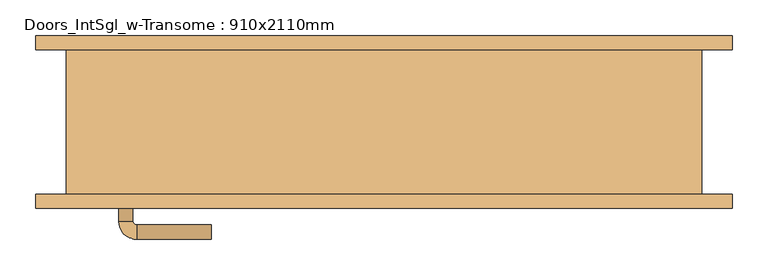
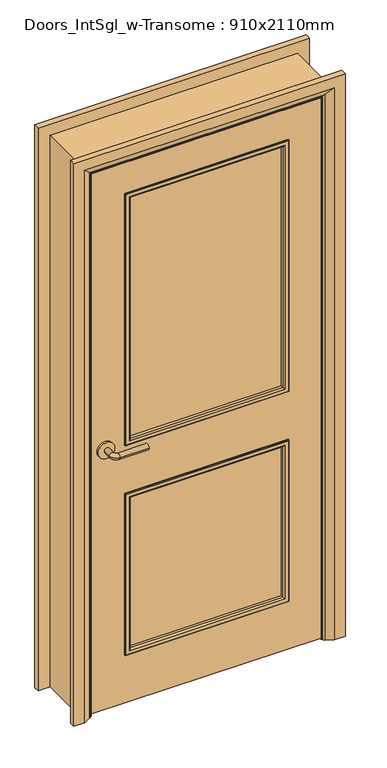
"""IFC4 building model written with IfcOpenShell, lengths in millimetres: door geometry, Doors_IntSgl_w-Transome : 910x2110mm."""

from ifc_helpers import new_model, si_unit, point, frame, frame_2d, origin, place, context, project, spatial, polyline, circle_curve, ellipse_curve, trimmed, segment, composite_curve, outline, extrude, faceted_brep, source, transform, mapped, element, save
from ifc_brep_helpers import plane_surface, cylinder_surface, revolved_surface, advanced_brep


def doors_intsgl_w_transome_910x2110mm_1071bad6(model_context):
    return source(origin(), model_context, "Body", "SolidModel", [
        advanced_brep(
        [(-373.0, -55.6, 1000.0), (-353.0, -55.6, 1000.0), (-373.0, -25.6, 1000.0), (-353.0, -25.6, 1000.0), (-348.0, -20.6, 1000.0), (-348.0, -0.6, 1000.0), (-243.0, -0.6, 1000.0), (-243.0, -20.6, 1000.0)],
        [
            (0, 1, circle_curve(frame((-363.0, -55.6, 1000.0), z_axis=(0.0, -1.0, 0.0), x_axis=(1.0, 0.0, 0.0)), 10.0)),
            (1, 0, circle_curve(frame((-363.0, -55.6, 1000.0), z_axis=(0.0, -1.0, 0.0), x_axis=(1.0, 0.0, 0.0)), 10.0)),
            (0, 2),
            (2, 3, circle_curve(frame((-363.0, -25.6, 1000.0), z_axis=(0.0, -1.0, 0.0), x_axis=(1.0, 0.0, 0.0)), 10.0)),
            (3, 1),
            (3, 2, circle_curve(frame((-363.0, -25.6, 1000.0), z_axis=(0.0, -1.0, 0.0), x_axis=(1.0, 0.0, 0.0)), 10.0)),
            (4, 3, circle_curve(frame((-348.0, -25.6, 1000.0), z_axis=(0.0, 0.0, 1.0), x_axis=(-1.0, 0.0, 0.0)), 5.0)),
            (2, 5, circle_curve(frame((-348.0, -25.6, 1000.0), z_axis=(0.0, 0.0, -1.0), x_axis=(-1.0, 0.0, 0.0)), 25.0)),
            (5, 4, circle_curve(frame((-348.0, -10.6, 1000.0), z_axis=(-1.0, 0.0, 0.0), x_axis=(0.0, -1.0, 0.0)), 10.0)),
            (4, 5, circle_curve(frame((-348.0, -10.6, 1000.0), z_axis=(-1.0, 0.0, 0.0), x_axis=(0.0, -1.0, 0.0)), 10.0)),
            (6, 7, circle_curve(frame((-243.0, -10.6, 1000.0), z_axis=(1.0, 0.0, 0.0), x_axis=(0.0, -1.0, 0.0)), 10.0)),
            (7, 6, circle_curve(frame((-243.0, -10.6, 1000.0), z_axis=(1.0, 0.0, 0.0), x_axis=(0.0, -1.0, 0.0)), 10.0)),
            (5, 6),
            (7, 4),
        ],
        [
            plane_surface(frame((-363.0, -55.6, 1000.0), z_axis=(0.0, -1.0, 0.0), x_axis=(0.0, 0.0, 1.0))),
            cylinder_surface(frame((-363.0, -55.6, 1000.0), z_axis=(0.0, -1.0, 0.0), x_axis=(1.0, 0.0, 0.0)), 10.0),
            revolved_surface(trimmed(ellipse_curve(frame((-363.0, -25.6, 1000.0), z_axis=(0.0, -1.0, 0.0), x_axis=(1.0, 0.0, 0.0)), 10.0, 10.0), [point((-373.0, -25.6, 1000.0))], [point((-353.0, -25.6, 1000.0))], True, "CARTESIAN"), (-348.0, -25.6, 1000.0), (0.0, 0.0, -1.0)),
            revolved_surface(trimmed(ellipse_curve(frame((-363.0, -25.6, 1000.0), z_axis=(0.0, -1.0, 0.0), x_axis=(1.0, 0.0, 0.0)), 10.0, 10.0), [point((-353.0, -25.6, 1000.0))], [point((-373.0, -25.6, 1000.0))], True, "CARTESIAN"), (-348.0, -25.6, 1000.0), (0.0, 0.0, -1.0)),
            plane_surface(frame((-243.0, -10.6, 1000.0), z_axis=(1.0, 0.0, 0.0), x_axis=(0.0, 0.0, 1.0))),
            cylinder_surface(frame((-348.0, -10.6, 1000.0), z_axis=(-1.0, 0.0, 0.0), x_axis=(0.0, -1.0, 0.0)), 10.0),
        ],
        [
            (0, [[1, 2]]),
            (1, [[-1, 3, 4, 5]]),
            (1, [[-2, -5, 6, -3]]),
            (2, [[7, -4, 8, 9]]),
            (3, [[-8, -6, -7, 10]]),
            (4, [[11, 12]]),
            (5, [[-9, 13, -12, 14]]),
            (5, [[-10, -14, -11, -13]]),
        ],
    ),
        extrude(outline(composite_curve([segment(trimmed(circle_curve(frame_2d((1000.0, -365.5)), 30.0), [point((1000.0, -395.5))], [point((1000.0, -335.5))], False, "CARTESIAN"), True, "CONTINUOUS"), segment(trimmed(circle_curve(frame_2d((1000.0, -365.5)), 30.0), [point((1000.0, -335.5))], [point((1000.0, -395.5))], False, "CARTESIAN"), True, "CONTINUOUS")], self_intersect=False)), frame((0.0, -63.6, 0.0), z_axis=(0.0, 1.0, 0.0), x_axis=(0.0, 0.0, 1.0)), (0.0, 0.0, 1.0), 8.0),
        advanced_brep(
        [(-373.0, -109.6, 1000.0), (-353.0, -109.6, 1000.0), (-353.0, -139.6, 1000.0), (-373.0, -139.6, 1000.0), (-348.0, -144.6, 1000.0), (-348.0, -164.6, 1000.0), (-243.0, -164.6, 1000.0), (-243.0, -144.6, 1000.0)],
        [
            (0, 1, circle_curve(frame((-363.0, -109.6, 1000.0), z_axis=(0.0, 1.0, 0.0), x_axis=(1.0, 0.0, 0.0)), 10.0)),
            (1, 0, circle_curve(frame((-363.0, -109.6, 1000.0), z_axis=(0.0, 1.0, 0.0), x_axis=(1.0, 0.0, 0.0)), 10.0)),
            (1, 2),
            (2, 3, circle_curve(frame((-363.0, -139.6, 1000.0), z_axis=(0.0, 1.0, 0.0), x_axis=(1.0, 0.0, 0.0)), 10.0)),
            (3, 0),
            (3, 2, circle_curve(frame((-363.0, -139.6, 1000.0), z_axis=(0.0, 1.0, 0.0), x_axis=(1.0, 0.0, 0.0)), 10.0)),
            (4, 5, circle_curve(frame((-348.0, -154.6, 1000.0), z_axis=(-1.0, 0.0, 0.0), x_axis=(0.0, 1.0, 0.0)), 10.0)),
            (5, 3, circle_curve(frame((-348.0, -139.6, 1000.0), z_axis=(0.0, 0.0, -1.0), x_axis=(-1.0, 0.0, 0.0)), 25.0)),
            (2, 4, circle_curve(frame((-348.0, -139.6, 1000.0), z_axis=(0.0, 0.0, 1.0), x_axis=(-1.0, 0.0, 0.0)), 5.0)),
            (5, 4, circle_curve(frame((-348.0, -154.6, 1000.0), z_axis=(-1.0, 0.0, 0.0), x_axis=(0.0, 1.0, 0.0)), 10.0)),
            (6, 7, circle_curve(frame((-243.0, -154.6, 1000.0), z_axis=(1.0, 0.0, 0.0), x_axis=(0.0, 1.0, 0.0)), 10.0)),
            (7, 6, circle_curve(frame((-243.0, -154.6, 1000.0), z_axis=(1.0, 0.0, 0.0), x_axis=(0.0, 1.0, 0.0)), 10.0)),
            (4, 7),
            (6, 5),
        ],
        [
            plane_surface(frame((-363.0, -109.6, 1000.0), z_axis=(0.0, 1.0, 0.0), x_axis=(0.0, 0.0, 1.0))),
            cylinder_surface(frame((-363.0, -109.6, 1000.0), z_axis=(0.0, 1.0, 0.0), x_axis=(1.0, 0.0, 0.0)), 10.0),
            revolved_surface(trimmed(ellipse_curve(frame((-363.0, -139.6, 1000.0), z_axis=(0.0, -1.0, 0.0), x_axis=(1.0, 0.0, 0.0)), 10.0, 10.0), [point((-373.0, -139.6, 1000.0))], [point((-353.0, -139.6, 1000.0))], True, "CARTESIAN"), (-348.0, -139.6, 1000.0), (0.0, 0.0, -1.0)),
            revolved_surface(trimmed(ellipse_curve(frame((-363.0, -139.6, 1000.0), z_axis=(0.0, -1.0, 0.0), x_axis=(1.0, 0.0, 0.0)), 10.0, 10.0), [point((-353.0, -139.6, 1000.0))], [point((-373.0, -139.6, 1000.0))], True, "CARTESIAN"), (-348.0, -139.6, 1000.0), (0.0, 0.0, -1.0)),
            plane_surface(frame((-243.0, -154.6, 1000.0), z_axis=(1.0, 0.0, 0.0), x_axis=(0.0, 0.0, 1.0))),
            cylinder_surface(frame((-348.0, -154.6, 1000.0), z_axis=(-1.0, 0.0, 0.0), x_axis=(0.0, 1.0, 0.0)), 10.0),
        ],
        [
            (0, [[1, 2]]),
            (1, [[3, 4, 5, -2]]),
            (1, [[-5, 6, -3, -1]]),
            (2, [[7, 8, -4, 9]]),
            (3, [[10, -9, -6, -8]]),
            (4, [[11, 12]]),
            (5, [[13, -11, 14, -7]]),
            (5, [[-14, -12, -13, -10]]),
        ],
    ),
        extrude(outline(composite_curve([segment(trimmed(circle_curve(frame_2d((1000.0, -365.5)), 30.0), [point((1000.0, -395.5))], [point((1000.0, -335.5))], False, "CARTESIAN"), True, "CONTINUOUS"), segment(trimmed(circle_curve(frame_2d((1000.0, -365.5)), 30.0), [point((1000.0, -335.5))], [point((1000.0, -395.5))], False, "CARTESIAN"), True, "CONTINUOUS")], self_intersect=False)), frame((0.0, -109.6, 0.0), z_axis=(0.0, 1.0, 0.0), x_axis=(0.0, 0.0, 1.0)), (0.0, 0.0, 1.0), 8.0),
        extrude(outline(polyline([(2068.0, -413.0), (8.0, -413.0), (8.0, 413.0), (2068.0, 413.0), (2068.0, -413.0)]), holes=[polyline([(1943.0, 288.0), (1000.0, 288.0), (1000.0, -288.0), (1943.0, -288.0), (1943.0, 288.0)]), polyline([(800.0, -288.0), (800.0, 288.0), (200.0, 288.0), (200.0, -288.0), (800.0, -288.0)])]), frame((0.0, -101.6, 0.0), z_axis=(0.0, 1.0, 0.0), x_axis=(0.0, 0.0, 1.0)), (0.0, 0.0, 1.0), 38.0),
        extrude(outline(polyline([(-288.0, -91.6), (-288.0, -73.6), (288.0, -73.6), (288.0, -91.6), (-288.0, -91.6)])), frame((0.0, 0.0, 1000.0), z_axis=(0.0, 0.0, 1.0), x_axis=(1.0, 0.0, 0.0)), (0.0, 0.0, 1.0), 943.0),
        extrude(outline(polyline([(-288.0, -91.6), (-288.0, -73.6), (288.0, -73.6), (288.0, -91.6), (-288.0, -91.6)])), frame((0.0, 0.0, 200.0), z_axis=(0.0, 0.0, 1.0), x_axis=(1.0, 0.0, 0.0)), (0.0, 0.0, 1.0), 600.0),
        faceted_brep([(-415.0, -101.6, 0.0), (-447.0, -101.6, 0.0), (-447.0, 101.6, 0.0), (-415.0, 101.6, 0.0), (-415.0, 101.6, 2070.0), (-415.0, -101.6, 2070.0), (-447.0, 101.6, 2102.0), (-447.0, -101.6, 2102.0), (415.0, -101.6, 0.0), (415.0, 101.6, 0.0), (447.0, 101.6, 0.0), (447.0, -101.6, 0.0), (415.0, -101.6, 2070.0), (447.0, -101.6, 2102.0), (447.0, 101.6, 2102.0), (415.0, 101.6, 2070.0)], [[[0, 1, 2, 3]], [[3, 4, 5, 0]], [[2, 6, 4, 3]], [[1, 7, 6, 2]], [[0, 5, 7, 1]], [[8, 9, 10, 11]], [[12, 8, 11, 13]], [[13, 11, 10, 14]], [[14, 10, 9, 15]], [[15, 9, 8, 12]], [[4, 15, 12, 5]], [[6, 14, 15, 4]], [[7, 13, 14, 6]], [[5, 12, 13, 7]]]),
        extrude(outline(polyline([(0.0, -396.0), (2051.0, -396.0), (2051.0, 396.0), (0.0, 396.0), (0.0, 415.0), (2070.0, 415.0), (2070.0, -415.0), (0.0, -415.0), (0.0, -396.0)])), frame((0.0, -61.6, 0.0), z_axis=(0.0, 1.0, 0.0), x_axis=(0.0, 0.0, 1.0)), (0.0, 0.0, 1.0), 32.0),
        advanced_brep(
        [(-490.0, 121.6, 0.0), (-450.0, 121.6, 0.0), (-424.0, 107.6, 0.0), (-420.0, 101.6, 0.0), (-490.0, 101.6, 0.0), (-490.0, 101.6, 2145.0), (-490.0, 121.6, 2145.0), (-420.0, 101.6, 2075.0), (420.0, 101.6, 2075.0), (420.0, 101.6, 0.0), (490.0, 101.6, 0.0), (490.0, 101.6, 2145.0), (-424.0, 107.6, 2079.0), (-450.0, 121.6, 2105.0), (490.0, 121.6, 2145.0), (490.0, 121.6, 0.0), (450.0, 121.6, 0.0), (450.0, 121.6, 2105.0), (424.0, 107.6, 0.0), (424.0, 107.6, 2079.0)],
        [
            (0, 1),
            (1, 2),
            (2, 3, circle_curve(frame((-428.0, 100.6, 0.0), z_axis=(0.0, 0.0, -1.0), x_axis=(-1.0, 0.0, 0.0)), 8.0622577)),
            (3, 4),
            (4, 0),
            (4, 5),
            (5, 6),
            (6, 0),
            (3, 7),
            (7, 8),
            (8, 9),
            (9, 10),
            (10, 11),
            (11, 5),
            (2, 12),
            (12, 7, ellipse_curve(frame((-428.0, 100.6, 2083.0), z_axis=(-0.7071067811865475, 0.0, -0.7071067811865475), x_axis=(0.7071067811865474, 0.0, -0.7071067811865476)), 11.4017543, 8.0622577)),
            (1, 13),
            (13, 12),
            (6, 14),
            (14, 15),
            (15, 16),
            (16, 17),
            (17, 13),
            (10, 15),
            (14, 11),
            (9, 18, circle_curve(frame((428.0, 100.6, 0.0), z_axis=(0.0, 0.0, -1.0), x_axis=(1.0, 0.0, 0.0)), 8.0622577)),
            (18, 16),
            (19, 18),
            (8, 19, ellipse_curve(frame((428.0, 100.6, 2083.0), z_axis=(0.7071067811865475, 0.0, -0.7071067811865475), x_axis=(0.7071067811865474, 0.0, 0.7071067811865476)), 11.4017543, 8.0622577)),
            (19, 17),
            (12, 19),
        ],
        [
            plane_surface(frame((-420.0, 101.6, 0.0), z_axis=(0.0, 0.0, -1.0), x_axis=(0.0, 1.0, 0.0))),
            plane_surface(frame((-490.0, 121.6, 0.0), z_axis=(-1.0, 0.0, 0.0), x_axis=(0.0, 0.0, 1.0))),
            plane_surface(frame((-490.0, 101.6, 0.0), z_axis=(0.0, -1.0, 0.0), x_axis=(0.0, 0.0, 1.0))),
            cylinder_surface(frame((-428.0, 100.6, 0.0), z_axis=(0.0, 0.0, -1.0), x_axis=(-1.0, 0.0, 0.0)), 8.0622577),
            plane_surface(frame((-424.0, 107.6, 0.0), z_axis=(0.4740998230350183, 0.8804710999221749, 0.0), x_axis=(0.0, 0.0, 1.0))),
            plane_surface(frame((-450.0, 121.6, 0.0), z_axis=(0.0, 1.0, 0.0), x_axis=(0.0, 0.0, 1.0))),
            plane_surface(frame((490.0, 121.6, 2145.0), z_axis=(1.0, 0.0, 0.0), x_axis=(0.0, 0.0, -1.0))),
            plane_surface(frame((420.0, 101.6, 0.0), z_axis=(0.0, 0.0, -1.0), x_axis=(0.0, 1.0, 0.0))),
            cylinder_surface(frame((428.0, 100.6, 2075.0), z_axis=(0.0, 0.0, 1.0), x_axis=(1.0, 0.0, 0.0)), 8.0622577),
            plane_surface(frame((424.0, 107.6, 2079.0), z_axis=(-0.4740998230350183, 0.8804710999221749, 0.0), x_axis=(0.0, 0.0, -1.0))),
            plane_surface(frame((-490.0, 121.6, 2145.0), z_axis=(0.0, 0.0, 1.0), x_axis=(1.0, 0.0, 0.0))),
            cylinder_surface(frame((-420.0, 100.6, 2083.0), z_axis=(-1.0, 0.0, 0.0), x_axis=(0.0, 0.0, 1.0)), 8.0622577),
            plane_surface(frame((-424.0, 107.6, 2079.0), z_axis=(0.0, 0.8804710999221749, -0.4740998230350183), x_axis=(1.0, 0.0, 0.0))),
        ],
        [
            (0, [[1, 2, 3, 4, 5]]),
            (1, [[6, 7, 8, -5]]),
            (2, [[9, 10, 11, 12, 13, 14, -6, -4]]),
            (3, [[15, 16, -9, -3]]),
            (4, [[17, 18, -15, -2]]),
            (5, [[-8, 19, 20, 21, 22, 23, -17, -1]]),
            (6, [[-13, 24, -20, 25]]),
            (7, [[-24, -12, 26, 27, -21]]),
            (8, [[28, -26, -11, 29]]),
            (9, [[-22, -27, -28, 30]]),
            (10, [[-14, -25, -19, -7]]),
            (11, [[31, -29, -10, -16]]),
            (12, [[-23, -30, -31, -18]]),
        ],
    ),
        advanced_brep(
        [(490.0, -121.6, 0.0), (450.0, -121.6, 0.0), (424.0, -107.6, 0.0), (420.0, -101.6, 0.0), (490.0, -101.6, 0.0), (490.0, -101.6, 2145.0), (490.0, -121.6, 2145.0), (420.0, -101.6, 2075.0), (-420.0, -101.6, 2075.0), (-420.0, -101.6, 0.0), (-490.0, -101.6, 0.0), (-490.0, -101.6, 2145.0), (424.0, -107.6, 2079.0), (450.0, -121.6, 2105.0), (-490.0, -121.6, 2145.0), (-490.0, -121.6, 0.0), (-450.0, -121.6, 0.0), (-450.0, -121.6, 2105.0), (-424.0, -107.6, 0.0), (-424.0, -107.6, 2079.0)],
        [
            (0, 1),
            (1, 2),
            (2, 3, circle_curve(frame((428.0, -100.6, 0.0), z_axis=(0.0, 0.0, -1.0), x_axis=(1.0, 0.0, 0.0)), 8.0622577)),
            (3, 4),
            (4, 0),
            (4, 5),
            (5, 6),
            (6, 0),
            (3, 7),
            (7, 8),
            (8, 9),
            (9, 10),
            (10, 11),
            (11, 5),
            (2, 12),
            (12, 7, ellipse_curve(frame((428.0, -100.6, 2083.0), z_axis=(0.7071067811865475, 0.0, -0.7071067811865475), x_axis=(-0.7071067811865474, 0.0, -0.7071067811865476)), 11.4017543, 8.0622577)),
            (1, 13),
            (13, 12),
            (6, 14),
            (14, 15),
            (15, 16),
            (16, 17),
            (17, 13),
            (10, 15),
            (14, 11),
            (9, 18, circle_curve(frame((-428.0, -100.6, 0.0), z_axis=(0.0, 0.0, -1.0), x_axis=(-1.0, 0.0, 0.0)), 8.0622577)),
            (18, 16),
            (19, 18),
            (8, 19, ellipse_curve(frame((-428.0, -100.6, 2083.0), z_axis=(-0.7071067811865475, 0.0, -0.7071067811865475), x_axis=(-0.7071067811865474, 0.0, 0.7071067811865476)), 11.4017543, 8.0622577)),
            (19, 17),
            (12, 19),
        ],
        [
            plane_surface(frame((420.0, -101.6, 0.0), z_axis=(0.0, 0.0, -1.0), x_axis=(0.0, 1.0, 0.0))),
            plane_surface(frame((490.0, -121.6, 0.0), z_axis=(1.0, 0.0, 0.0), x_axis=(0.0, 0.0, 1.0))),
            plane_surface(frame((490.0, -101.6, 0.0), z_axis=(0.0, 1.0, 0.0), x_axis=(0.0, 0.0, 1.0))),
            cylinder_surface(frame((428.0, -100.6, 0.0), z_axis=(0.0, 0.0, -1.0), x_axis=(1.0, 0.0, 0.0)), 8.0622577),
            plane_surface(frame((424.0, -107.6, 0.0), z_axis=(-0.4740998230350126, -0.880471099922178, 0.0), x_axis=(0.0, 0.0, 1.0))),
            plane_surface(frame((450.0, -121.6, 0.0), z_axis=(0.0, -1.0, 0.0), x_axis=(0.0, 0.0, 1.0))),
            plane_surface(frame((-490.0, -121.6, 2145.0), z_axis=(-1.0, 0.0, 0.0), x_axis=(0.0, 0.0, -1.0))),
            plane_surface(frame((-420.0, -101.6, 0.0), z_axis=(0.0, 0.0, -1.0), x_axis=(0.0, 1.0, 0.0))),
            cylinder_surface(frame((-428.0, -100.6, 2075.0), z_axis=(0.0, 0.0, 1.0), x_axis=(-1.0, 0.0, 0.0)), 8.0622577),
            plane_surface(frame((-424.0, -107.6, 2079.0), z_axis=(0.47409982303501824, -0.8804710999221749, 0.0), x_axis=(0.0, 0.0, -1.0))),
            plane_surface(frame((490.0, -121.6, 2145.0), z_axis=(0.0, 0.0, 1.0), x_axis=(-1.0, 0.0, 0.0))),
            cylinder_surface(frame((420.0, -100.6, 2083.0), z_axis=(1.0, 0.0, 0.0), x_axis=(0.0, 0.0, 1.0)), 8.0622577),
            plane_surface(frame((424.0, -107.6, 2079.0), z_axis=(0.0, -0.8804710999221764, -0.4740998230350154), x_axis=(-1.0, 0.0, 0.0))),
        ],
        [
            (0, [[1, 2, 3, 4, 5]]),
            (1, [[6, 7, 8, -5]]),
            (2, [[9, 10, 11, 12, 13, 14, -6, -4]]),
            (3, [[15, 16, -9, -3]]),
            (4, [[17, 18, -15, -2]]),
            (5, [[-8, 19, 20, 21, 22, 23, -17, -1]]),
            (6, [[-13, 24, -20, 25]]),
            (7, [[-24, -12, 26, 27, -21]]),
            (8, [[28, -26, -11, 29]]),
            (9, [[-22, -27, -28, 30]]),
            (10, [[-14, -25, -19, -7]]),
            (11, [[31, -29, -10, -16]]),
            (12, [[-23, -30, -31, -18]]),
        ],
    ),
        advanced_brep(
        [(-288.0, -91.6, 1943.0), (-288.0, -91.6, 1000.0), (-288.0, -101.6, 1000.0), (-288.0, -101.6, 1943.0), (-276.0, -102.6, 1931.0), (-276.0, -102.6, 1012.0), (-276.0, -91.6, 1012.0), (-276.0, -91.6, 1931.0), (-281.0, -107.6, 1936.0), (-281.0, -107.6, 1007.0), (-296.0, -105.6, 1951.0), (-296.0, -105.6, 992.0), (-294.0, -107.6, 994.0), (-294.0, -107.6, 1949.0), (-296.0, -101.6, 1951.0), (-296.0, -101.6, 992.0), (288.0, -91.6, 1000.0), (288.0, -101.6, 1000.0), (276.0, -102.6, 1012.0), (276.0, -91.6, 1012.0), (281.0, -107.6, 1007.0), (296.0, -105.6, 992.0), (294.0, -107.6, 994.0), (296.0, -101.6, 992.0), (288.0, -91.6, 1943.0), (288.0, -101.6, 1943.0), (276.0, -102.6, 1931.0), (276.0, -91.6, 1931.0), (281.0, -107.6, 1936.0), (296.0, -105.6, 1951.0), (294.0, -107.6, 1949.0), (296.0, -101.6, 1951.0)],
        [
            (0, 1),
            (1, 2),
            (2, 3),
            (3, 0),
            (4, 5),
            (5, 6),
            (6, 7),
            (7, 4),
            (8, 9),
            (9, 5, ellipse_curve(frame((-281.0, -102.6, 1007.0), z_axis=(-0.7071067811865475, 0.0, 0.7071067811865475), x_axis=(0.7071067811865474, 0.0, 0.7071067811865476)), 7.0710678, 5.0)),
            (4, 8, ellipse_curve(frame((-281.0, -102.6, 1936.0), z_axis=(-0.7071067811865475, 0.0, -0.7071067811865475), x_axis=(-0.7071067811865474, 0.0, 0.7071067811865476)), 7.0710678, 5.0)),
            (10, 11),
            (11, 12, ellipse_curve(frame((-294.0, -105.6, 994.0), z_axis=(-0.7071067811865475, 0.0, 0.7071067811865475), x_axis=(0.7071067811865474, 0.0, 0.7071067811865476)), 2.8284271, 2.0)),
            (12, 13),
            (13, 10, ellipse_curve(frame((-294.0, -105.6, 1949.0), z_axis=(-0.7071067811865475, 0.0, -0.7071067811865475), x_axis=(-0.7071067811865474, 0.0, 0.7071067811865476)), 2.8284271, 2.0)),
            (14, 15),
            (15, 11),
            (10, 14),
            (1, 16),
            (16, 17),
            (17, 2),
            (5, 18),
            (18, 19),
            (19, 6),
            (9, 20),
            (20, 18, ellipse_curve(frame((281.0, -102.6, 1007.0), z_axis=(-0.7071067811865475, 0.0, -0.7071067811865475), x_axis=(-0.7071067811865476, 0.0, 0.7071067811865474)), 7.0710678, 5.0)),
            (11, 21),
            (21, 22, ellipse_curve(frame((294.0, -105.6, 994.0), z_axis=(-0.7071067811865475, 0.0, -0.7071067811865475), x_axis=(-0.7071067811865476, 0.0, 0.7071067811865474)), 2.8284271, 2.0)),
            (22, 12),
            (15, 23),
            (23, 21),
            (16, 24),
            (24, 25),
            (25, 17),
            (18, 26),
            (26, 27),
            (27, 19),
            (20, 28),
            (28, 26, ellipse_curve(frame((281.0, -102.6, 1936.0), z_axis=(0.7071067811865475, 0.0, -0.7071067811865475), x_axis=(-0.7071067811865474, 0.0, -0.7071067811865476)), 7.0710678, 5.0)),
            (21, 29),
            (29, 30, ellipse_curve(frame((294.0, -105.6, 1949.0), z_axis=(0.7071067811865475, 0.0, -0.7071067811865475), x_axis=(-0.7071067811865474, 0.0, -0.7071067811865476)), 2.8284271, 2.0)),
            (30, 22),
            (23, 31),
            (31, 29),
            (14, 31),
            (25, 3),
            (24, 0),
            (27, 7),
            (26, 4),
            (28, 8),
            (30, 13),
            (29, 10),
        ],
        [
            plane_surface(frame((-288.0, -101.6, 1943.0), z_axis=(-1.0, 0.0, 0.0), x_axis=(0.0, 0.0, -1.0))),
            plane_surface(frame((-276.0, -91.6, 1931.0), z_axis=(1.0, 0.0, 0.0), x_axis=(0.0, 0.0, -1.0))),
            cylinder_surface(frame((-281.0, -102.6, 1943.0), z_axis=(0.0, 0.0, 1.0), x_axis=(-1.0, 0.0, 0.0)), 5.0),
            cylinder_surface(frame((-294.0, -105.6, 1943.0), z_axis=(0.0, 0.0, 1.0), x_axis=(-1.0, 0.0, 0.0)), 2.0),
            plane_surface(frame((-296.0, -105.6, 1951.0), z_axis=(-1.0, 0.0, 0.0), x_axis=(0.0, 0.0, -1.0))),
            plane_surface(frame((-288.0, -101.6, 1000.0), z_axis=(0.0, 0.0, -1.0), x_axis=(1.0, 0.0, 0.0))),
            plane_surface(frame((-276.0, -91.6, 1012.0), z_axis=(0.0, 0.0, 1.0), x_axis=(1.0, 0.0, 0.0))),
            cylinder_surface(frame((-288.0, -102.6, 1007.0), z_axis=(-1.0, 0.0, 0.0), x_axis=(0.0, 0.0, -1.0)), 5.0),
            cylinder_surface(frame((-288.0, -105.6, 994.0), z_axis=(-1.0, 0.0, 0.0), x_axis=(0.0, 0.0, -1.0)), 2.0),
            plane_surface(frame((-296.0, -105.6, 992.0), z_axis=(0.0, 0.0, -1.0), x_axis=(1.0, 0.0, 0.0))),
            plane_surface(frame((288.0, -101.6, 1000.0), z_axis=(1.0, 0.0, 0.0), x_axis=(0.0, 0.0, 1.0))),
            plane_surface(frame((276.0, -91.6, 1012.0), z_axis=(-1.0, 0.0, 0.0), x_axis=(0.0, 0.0, 1.0))),
            cylinder_surface(frame((281.0, -102.6, 1000.0), z_axis=(0.0, 0.0, -1.0), x_axis=(1.0, 0.0, 0.0)), 5.0),
            cylinder_surface(frame((294.0, -105.6, 1000.0), z_axis=(0.0, 0.0, -1.0), x_axis=(1.0, 0.0, 0.0)), 2.0),
            plane_surface(frame((296.0, -105.6, 992.0), z_axis=(1.0, 0.0, 0.0), x_axis=(0.0, 0.0, 1.0))),
            plane_surface(frame((296.0, -101.6, 1951.0), z_axis=(0.0, 1.0, 0.0), x_axis=(-1.0, 0.0, 0.0))),
            plane_surface(frame((288.0, -101.6, 1943.0), z_axis=(0.0, 0.0, 1.0), x_axis=(-1.0, 0.0, 0.0))),
            plane_surface(frame((288.0, -91.6, 1943.0), z_axis=(0.0, 1.0, 0.0), x_axis=(-1.0, 0.0, 0.0))),
            plane_surface(frame((276.0, -91.6, 1931.0), z_axis=(0.0, 0.0, -1.0), x_axis=(-1.0, 0.0, 0.0))),
            cylinder_surface(frame((288.0, -102.6, 1936.0), z_axis=(1.0, 0.0, 0.0), x_axis=(0.0, 0.0, 1.0)), 5.0),
            plane_surface(frame((281.0, -107.6, 1936.0), z_axis=(0.0, -1.0, 0.0), x_axis=(-1.0, 0.0, 0.0))),
            cylinder_surface(frame((288.0, -105.6, 1949.0), z_axis=(1.0, 0.0, 0.0), x_axis=(0.0, 0.0, 1.0)), 2.0),
            plane_surface(frame((296.0, -105.6, 1951.0), z_axis=(0.0, 0.0, 1.0), x_axis=(-1.0, 0.0, 0.0))),
        ],
        [
            (0, [[1, 2, 3, 4]]),
            (1, [[5, 6, 7, 8]]),
            (2, [[9, 10, -5, 11]]),
            (3, [[12, 13, 14, 15]]),
            (4, [[16, 17, -12, 18]]),
            (5, [[19, 20, 21, -2]]),
            (6, [[22, 23, 24, -6]]),
            (7, [[25, 26, -22, -10]]),
            (8, [[27, 28, 29, -13]]),
            (9, [[30, 31, -27, -17]]),
            (10, [[32, 33, 34, -20]]),
            (11, [[35, 36, 37, -23]]),
            (12, [[38, 39, -35, -26]]),
            (13, [[40, 41, 42, -28]]),
            (14, [[43, 44, -40, -31]]),
            (15, [[-16, 45, -43, -30], [-3, -21, -34, 46]]),
            (16, [[47, -4, -46, -33]]),
            (17, [[-1, -47, -32, -19], [-7, -24, -37, 48]]),
            (18, [[49, -8, -48, -36]]),
            (19, [[50, -11, -49, -39]]),
            (20, [[-14, -29, -42, 51], [-9, -50, -38, -25]]),
            (21, [[52, -15, -51, -41]]),
            (22, [[-45, -18, -52, -44]]),
        ],
    ),
        advanced_brep(
        [(288.0, -73.6, 1943.0), (288.0, -73.6, 1000.0), (288.0, -63.6, 1000.0), (288.0, -63.6, 1943.0), (276.0, -62.6, 1931.0), (276.0, -62.6, 1012.0), (276.0, -73.6, 1012.0), (276.0, -73.6, 1931.0), (281.0, -57.6, 1936.0), (281.0, -57.6, 1007.0), (296.0, -59.6, 1951.0), (296.0, -59.6, 992.0), (294.0, -57.6, 994.0), (294.0, -57.6, 1949.0), (296.0, -63.6, 1951.0), (296.0, -63.6, 992.0), (-288.0, -73.6, 1000.0), (-288.0, -63.6, 1000.0), (-276.0, -62.6, 1012.0), (-276.0, -73.6, 1012.0), (-281.0, -57.6, 1007.0), (-296.0, -59.6, 992.0), (-294.0, -57.6, 994.0), (-296.0, -63.6, 992.0), (-288.0, -73.6, 1943.0), (-288.0, -63.6, 1943.0), (-276.0, -62.6, 1931.0), (-276.0, -73.6, 1931.0), (-281.0, -57.6, 1936.0), (-296.0, -59.6, 1951.0), (-294.0, -57.6, 1949.0), (-296.0, -63.6, 1951.0)],
        [
            (0, 1),
            (1, 2),
            (2, 3),
            (3, 0),
            (4, 5),
            (5, 6),
            (6, 7),
            (7, 4),
            (8, 9),
            (9, 5, ellipse_curve(frame((281.0, -62.6, 1007.0), z_axis=(0.7071067811865475, 0.0, 0.7071067811865475), x_axis=(-0.7071067811865474, 0.0, 0.7071067811865476)), 7.0710678, 5.0)),
            (4, 8, ellipse_curve(frame((281.0, -62.6, 1936.0), z_axis=(0.7071067811865475, 0.0, -0.7071067811865475), x_axis=(0.7071067811865474, 0.0, 0.7071067811865476)), 7.0710678, 5.0)),
            (10, 11),
            (11, 12, ellipse_curve(frame((294.0, -59.6, 994.0), z_axis=(0.7071067811865475, 0.0, 0.7071067811865475), x_axis=(-0.7071067811865474, 0.0, 0.7071067811865476)), 2.8284271, 2.0)),
            (12, 13),
            (13, 10, ellipse_curve(frame((294.0, -59.6, 1949.0), z_axis=(0.7071067811865475, 0.0, -0.7071067811865475), x_axis=(0.7071067811865474, 0.0, 0.7071067811865476)), 2.8284271, 2.0)),
            (14, 15),
            (15, 11),
            (10, 14),
            (1, 16),
            (16, 17),
            (17, 2),
            (5, 18),
            (18, 19),
            (19, 6),
            (9, 20),
            (20, 18, ellipse_curve(frame((-281.0, -62.6, 1007.0), z_axis=(0.7071067811865475, 0.0, -0.7071067811865475), x_axis=(0.7071067811865476, 0.0, 0.7071067811865474)), 7.0710678, 5.0)),
            (11, 21),
            (21, 22, ellipse_curve(frame((-294.0, -59.6, 994.0), z_axis=(0.7071067811865475, 0.0, -0.7071067811865475), x_axis=(0.7071067811865476, 0.0, 0.7071067811865474)), 2.8284271, 2.0)),
            (22, 12),
            (15, 23),
            (23, 21),
            (16, 24),
            (24, 25),
            (25, 17),
            (18, 26),
            (26, 27),
            (27, 19),
            (20, 28),
            (28, 26, ellipse_curve(frame((-281.0, -62.6, 1936.0), z_axis=(-0.7071067811865475, 0.0, -0.7071067811865475), x_axis=(0.7071067811865474, 0.0, -0.7071067811865476)), 7.0710678, 5.0)),
            (21, 29),
            (29, 30, ellipse_curve(frame((-294.0, -59.6, 1949.0), z_axis=(-0.7071067811865475, 0.0, -0.7071067811865475), x_axis=(0.7071067811865474, 0.0, -0.7071067811865476)), 2.8284271, 2.0)),
            (30, 22),
            (23, 31),
            (31, 29),
            (14, 31),
            (25, 3),
            (24, 0),
            (27, 7),
            (26, 4),
            (28, 8),
            (30, 13),
            (29, 10),
        ],
        [
            plane_surface(frame((288.0, -63.6, 1943.0), z_axis=(1.0, 0.0, 0.0), x_axis=(0.0, 0.0, -1.0))),
            plane_surface(frame((276.0, -73.6, 1931.0), z_axis=(-1.0, 0.0, 0.0), x_axis=(0.0, 0.0, -1.0))),
            cylinder_surface(frame((281.0, -62.6, 1943.0), z_axis=(0.0, 0.0, 1.0), x_axis=(1.0, 0.0, 0.0)), 5.0),
            cylinder_surface(frame((294.0, -59.6, 1943.0), z_axis=(0.0, 0.0, 1.0), x_axis=(1.0, 0.0, 0.0)), 2.0),
            plane_surface(frame((296.0, -59.6, 1951.0), z_axis=(1.0, 0.0, 0.0), x_axis=(0.0, 0.0, -1.0))),
            plane_surface(frame((288.0, -63.6, 1000.0), z_axis=(0.0, 0.0, -1.0), x_axis=(-1.0, 0.0, 0.0))),
            plane_surface(frame((276.0, -73.6, 1012.0), z_axis=(0.0, 0.0, 1.0), x_axis=(-1.0, 0.0, 0.0))),
            cylinder_surface(frame((288.0, -62.6, 1007.0), z_axis=(1.0, 0.0, 0.0), x_axis=(0.0, 0.0, -1.0)), 5.0),
            cylinder_surface(frame((288.0, -59.6, 994.0), z_axis=(1.0, 0.0, 0.0), x_axis=(0.0, 0.0, -1.0)), 2.0),
            plane_surface(frame((296.0, -59.6, 992.0), z_axis=(0.0, 0.0, -1.0), x_axis=(-1.0, 0.0, 0.0))),
            plane_surface(frame((-288.0, -63.6, 1000.0), z_axis=(-1.0, 0.0, 0.0), x_axis=(0.0, 0.0, 1.0))),
            plane_surface(frame((-276.0, -73.6, 1012.0), z_axis=(1.0, 0.0, 0.0), x_axis=(0.0, 0.0, 1.0))),
            cylinder_surface(frame((-281.0, -62.6, 1000.0), z_axis=(0.0, 0.0, -1.0), x_axis=(-1.0, 0.0, 0.0)), 5.0),
            cylinder_surface(frame((-294.0, -59.6, 1000.0), z_axis=(0.0, 0.0, -1.0), x_axis=(-1.0, 0.0, 0.0)), 2.0),
            plane_surface(frame((-296.0, -59.6, 992.0), z_axis=(-1.0, 0.0, 0.0), x_axis=(0.0, 0.0, 1.0))),
            plane_surface(frame((-296.0, -63.6, 1951.0), z_axis=(0.0, -1.0, 0.0), x_axis=(1.0, 0.0, 0.0))),
            plane_surface(frame((-288.0, -63.6, 1943.0), z_axis=(0.0, 0.0, 1.0), x_axis=(1.0, 0.0, 0.0))),
            plane_surface(frame((-288.0, -73.6, 1943.0), z_axis=(0.0, -1.0, 0.0), x_axis=(1.0, 0.0, 0.0))),
            plane_surface(frame((-276.0, -73.6, 1931.0), z_axis=(0.0, 0.0, -1.0), x_axis=(1.0, 0.0, 0.0))),
            cylinder_surface(frame((-288.0, -62.6, 1936.0), z_axis=(-1.0, 0.0, 0.0), x_axis=(0.0, 0.0, 1.0)), 5.0),
            plane_surface(frame((-281.0, -57.6, 1936.0), z_axis=(0.0, 1.0, 0.0), x_axis=(1.0, 0.0, 0.0))),
            cylinder_surface(frame((-288.0, -59.6, 1949.0), z_axis=(-1.0, 0.0, 0.0), x_axis=(0.0, 0.0, 1.0)), 2.0),
            plane_surface(frame((-296.0, -59.6, 1951.0), z_axis=(0.0, 0.0, 1.0), x_axis=(1.0, 0.0, 0.0))),
        ],
        [
            (0, [[1, 2, 3, 4]]),
            (1, [[5, 6, 7, 8]]),
            (2, [[9, 10, -5, 11]]),
            (3, [[12, 13, 14, 15]]),
            (4, [[16, 17, -12, 18]]),
            (5, [[19, 20, 21, -2]]),
            (6, [[22, 23, 24, -6]]),
            (7, [[25, 26, -22, -10]]),
            (8, [[27, 28, 29, -13]]),
            (9, [[30, 31, -27, -17]]),
            (10, [[32, 33, 34, -20]]),
            (11, [[35, 36, 37, -23]]),
            (12, [[38, 39, -35, -26]]),
            (13, [[40, 41, 42, -28]]),
            (14, [[43, 44, -40, -31]]),
            (15, [[-16, 45, -43, -30], [-3, -21, -34, 46]]),
            (16, [[47, -4, -46, -33]]),
            (17, [[-1, -47, -32, -19], [-7, -24, -37, 48]]),
            (18, [[49, -8, -48, -36]]),
            (19, [[50, -11, -49, -39]]),
            (20, [[-14, -29, -42, 51], [-9, -50, -38, -25]]),
            (21, [[52, -15, -51, -41]]),
            (22, [[-45, -18, -52, -44]]),
        ],
    ),
        advanced_brep(
        [(296.0, -105.6, 808.0), (296.0, -105.6, 192.0), (296.0, -101.6, 192.0), (296.0, -101.6, 808.0), (294.0, -107.6, 806.0), (294.0, -107.6, 194.0), (276.0, -102.6, 788.0), (276.0, -102.6, 212.0), (281.0, -107.6, 207.0), (281.0, -107.6, 793.0), (276.0, -91.6, 788.0), (276.0, -91.6, 212.0), (288.0, -101.6, 800.0), (288.0, -101.6, 200.0), (288.0, -91.6, 200.0), (288.0, -91.6, 800.0), (-296.0, -105.6, 192.0), (-296.0, -101.6, 192.0), (-294.0, -107.6, 194.0), (-276.0, -102.6, 212.0), (-281.0, -107.6, 207.0), (-276.0, -91.6, 212.0), (-288.0, -101.6, 200.0), (-288.0, -91.6, 200.0), (-296.0, -105.6, 808.0), (-296.0, -101.6, 808.0), (-294.0, -107.6, 806.0), (-276.0, -102.6, 788.0), (-281.0, -107.6, 793.0), (-276.0, -91.6, 788.0), (-288.0, -101.6, 800.0), (-288.0, -91.6, 800.0)],
        [
            (0, 1),
            (1, 2),
            (2, 3),
            (3, 0),
            (4, 5),
            (5, 1, ellipse_curve(frame((294.0, -105.6, 194.0), z_axis=(0.7071067811865475, 0.0, 0.7071067811865475), x_axis=(-0.7071067811865474, 0.0, 0.7071067811865476)), 2.8284271, 2.0)),
            (0, 4, ellipse_curve(frame((294.0, -105.6, 806.0), z_axis=(0.7071067811865475, 0.0, -0.7071067811865475), x_axis=(0.7071067811865474, 0.0, 0.7071067811865476)), 2.8284271, 2.0)),
            (6, 7),
            (7, 8, ellipse_curve(frame((281.0, -102.6, 207.0), z_axis=(0.7071067811865475, 0.0, 0.7071067811865475), x_axis=(-0.7071067811865474, 0.0, 0.7071067811865476)), 7.0710678, 5.0)),
            (8, 9),
            (9, 6, ellipse_curve(frame((281.0, -102.6, 793.0), z_axis=(0.7071067811865475, 0.0, -0.7071067811865475), x_axis=(0.7071067811865474, 0.0, 0.7071067811865476)), 7.0710678, 5.0)),
            (10, 11),
            (11, 7),
            (6, 10),
            (12, 13),
            (13, 14),
            (14, 15),
            (15, 12),
            (1, 16),
            (16, 17),
            (17, 2),
            (5, 18),
            (18, 16, ellipse_curve(frame((-294.0, -105.6, 194.0), z_axis=(0.7071067811865475, 0.0, -0.7071067811865475), x_axis=(0.7071067811865476, 0.0, 0.7071067811865474)), 2.8284271, 2.0)),
            (7, 19),
            (19, 20, ellipse_curve(frame((-281.0, -102.6, 207.0), z_axis=(0.7071067811865475, 0.0, -0.7071067811865475), x_axis=(0.7071067811865476, 0.0, 0.7071067811865474)), 7.0710678, 5.0)),
            (20, 8),
            (11, 21),
            (21, 19),
            (13, 22),
            (22, 23),
            (23, 14),
            (16, 24),
            (24, 25),
            (25, 17),
            (18, 26),
            (26, 24, ellipse_curve(frame((-294.0, -105.6, 806.0), z_axis=(-0.7071067811865475, 0.0, -0.7071067811865475), x_axis=(0.7071067811865474, 0.0, -0.7071067811865476)), 2.8284271, 2.0)),
            (19, 27),
            (27, 28, ellipse_curve(frame((-281.0, -102.6, 793.0), z_axis=(-0.7071067811865475, 0.0, -0.7071067811865475), x_axis=(0.7071067811865474, 0.0, -0.7071067811865476)), 7.0710678, 5.0)),
            (28, 20),
            (21, 29),
            (29, 27),
            (22, 30),
            (30, 31),
            (31, 23),
            (24, 0),
            (3, 25),
            (26, 4),
            (28, 9),
            (27, 6),
            (29, 10),
            (31, 15),
            (30, 12),
        ],
        [
            plane_surface(frame((296.0, -101.6, 808.0), z_axis=(1.0, 0.0, 0.0), x_axis=(0.0, 0.0, -1.0))),
            cylinder_surface(frame((294.0, -105.6, 800.0), z_axis=(0.0, 0.0, 1.0), x_axis=(1.0, 0.0, 0.0)), 2.0),
            cylinder_surface(frame((281.0, -102.6, 800.0), z_axis=(0.0, 0.0, 1.0), x_axis=(1.0, 0.0, 0.0)), 5.0),
            plane_surface(frame((276.0, -102.6, 788.0), z_axis=(-1.0, 0.0, 0.0), x_axis=(0.0, 0.0, -1.0))),
            plane_surface(frame((288.0, -91.6, 800.0), z_axis=(1.0, 0.0, 0.0), x_axis=(0.0, 0.0, -1.0))),
            plane_surface(frame((296.0, -101.6, 192.0), z_axis=(0.0, 0.0, -1.0), x_axis=(-1.0, 0.0, 0.0))),
            cylinder_surface(frame((288.0, -105.6, 194.0), z_axis=(1.0, 0.0, 0.0), x_axis=(0.0, 0.0, -1.0)), 2.0),
            cylinder_surface(frame((288.0, -102.6, 207.0), z_axis=(1.0, 0.0, 0.0), x_axis=(0.0, 0.0, -1.0)), 5.0),
            plane_surface(frame((276.0, -102.6, 212.0), z_axis=(0.0, 0.0, 1.0), x_axis=(-1.0, 0.0, 0.0))),
            plane_surface(frame((288.0, -91.6, 200.0), z_axis=(0.0, 0.0, -1.0), x_axis=(-1.0, 0.0, 0.0))),
            plane_surface(frame((-296.0, -101.6, 192.0), z_axis=(-1.0, 0.0, 0.0), x_axis=(0.0, 0.0, 1.0))),
            cylinder_surface(frame((-294.0, -105.6, 200.0), z_axis=(0.0, 0.0, -1.0), x_axis=(-1.0, 0.0, 0.0)), 2.0),
            cylinder_surface(frame((-281.0, -102.6, 200.0), z_axis=(0.0, 0.0, -1.0), x_axis=(-1.0, 0.0, 0.0)), 5.0),
            plane_surface(frame((-276.0, -102.6, 212.0), z_axis=(1.0, 0.0, 0.0), x_axis=(0.0, 0.0, 1.0))),
            plane_surface(frame((-288.0, -91.6, 200.0), z_axis=(-1.0, 0.0, 0.0), x_axis=(0.0, 0.0, 1.0))),
            plane_surface(frame((-296.0, -101.6, 808.0), z_axis=(0.0, 0.0, 1.0), x_axis=(1.0, 0.0, 0.0))),
            cylinder_surface(frame((-288.0, -105.6, 806.0), z_axis=(-1.0, 0.0, 0.0), x_axis=(0.0, 0.0, 1.0)), 2.0),
            plane_surface(frame((-294.0, -107.6, 806.0), z_axis=(0.0, -1.0, 0.0), x_axis=(1.0, 0.0, 0.0))),
            cylinder_surface(frame((-288.0, -102.6, 793.0), z_axis=(-1.0, 0.0, 0.0), x_axis=(0.0, 0.0, 1.0)), 5.0),
            plane_surface(frame((-276.0, -102.6, 788.0), z_axis=(0.0, 0.0, -1.0), x_axis=(1.0, 0.0, 0.0))),
            plane_surface(frame((-276.0, -91.6, 788.0), z_axis=(0.0, 1.0, 0.0), x_axis=(1.0, 0.0, 0.0))),
            plane_surface(frame((-288.0, -91.6, 800.0), z_axis=(0.0, 0.0, 1.0), x_axis=(1.0, 0.0, 0.0))),
            plane_surface(frame((-288.0, -101.6, 800.0), z_axis=(0.0, 1.0, 0.0), x_axis=(1.0, 0.0, 0.0))),
        ],
        [
            (0, [[1, 2, 3, 4]]),
            (1, [[5, 6, -1, 7]]),
            (2, [[8, 9, 10, 11]]),
            (3, [[12, 13, -8, 14]]),
            (4, [[15, 16, 17, 18]]),
            (5, [[19, 20, 21, -2]]),
            (6, [[22, 23, -19, -6]]),
            (7, [[24, 25, 26, -9]]),
            (8, [[27, 28, -24, -13]]),
            (9, [[29, 30, 31, -16]]),
            (10, [[32, 33, 34, -20]]),
            (11, [[35, 36, -32, -23]]),
            (12, [[37, 38, 39, -25]]),
            (13, [[40, 41, -37, -28]]),
            (14, [[42, 43, 44, -30]]),
            (15, [[45, -4, 46, -33]]),
            (16, [[47, -7, -45, -36]]),
            (17, [[-5, -47, -35, -22], [-10, -26, -39, 48]]),
            (18, [[49, -11, -48, -38]]),
            (19, [[50, -14, -49, -41]]),
            (20, [[-17, -31, -44, 51], [-12, -50, -40, -27]]),
            (21, [[52, -18, -51, -43]]),
            (22, [[-3, -21, -34, -46], [-15, -52, -42, -29]]),
        ],
    ),
        advanced_brep(
        [(288.0, -73.6, 800.0), (288.0, -73.6, 200.0), (288.0, -63.6, 200.0), (288.0, -63.6, 800.0), (276.0, -62.6, 788.0), (276.0, -62.6, 212.0), (276.0, -73.6, 212.0), (276.0, -73.6, 788.0), (281.0, -57.6, 793.0), (281.0, -57.6, 207.0), (296.0, -59.6, 808.0), (296.0, -59.6, 192.0), (294.0, -57.6, 194.0), (294.0, -57.6, 806.0), (296.0, -63.6, 808.0), (296.0, -63.6, 192.0), (-288.0, -73.6, 200.0), (-288.0, -63.6, 200.0), (-276.0, -62.6, 212.0), (-276.0, -73.6, 212.0), (-281.0, -57.6, 207.0), (-296.0, -59.6, 192.0), (-294.0, -57.6, 194.0), (-296.0, -63.6, 192.0), (-288.0, -73.6, 800.0), (-288.0, -63.6, 800.0), (-276.0, -62.6, 788.0), (-276.0, -73.6, 788.0), (-281.0, -57.6, 793.0), (-296.0, -59.6, 808.0), (-294.0, -57.6, 806.0), (-296.0, -63.6, 808.0)],
        [
            (0, 1),
            (1, 2),
            (2, 3),
            (3, 0),
            (4, 5),
            (5, 6),
            (6, 7),
            (7, 4),
            (8, 9),
            (9, 5, ellipse_curve(frame((281.0, -62.6, 207.0), z_axis=(0.7071067811865475, 0.0, 0.7071067811865475), x_axis=(-0.7071067811865474, 0.0, 0.7071067811865476)), 7.0710678, 5.0)),
            (4, 8, ellipse_curve(frame((281.0, -62.6, 793.0), z_axis=(0.7071067811865475, 0.0, -0.7071067811865475), x_axis=(0.7071067811865474, 0.0, 0.7071067811865476)), 7.0710678, 5.0)),
            (10, 11),
            (11, 12, ellipse_curve(frame((294.0, -59.6, 194.0), z_axis=(0.7071067811865475, 0.0, 0.7071067811865475), x_axis=(-0.7071067811865474, 0.0, 0.7071067811865476)), 2.8284271, 2.0)),
            (12, 13),
            (13, 10, ellipse_curve(frame((294.0, -59.6, 806.0), z_axis=(0.7071067811865475, 0.0, -0.7071067811865475), x_axis=(0.7071067811865474, 0.0, 0.7071067811865476)), 2.8284271, 2.0)),
            (14, 15),
            (15, 11),
            (10, 14),
            (1, 16),
            (16, 17),
            (17, 2),
            (5, 18),
            (18, 19),
            (19, 6),
            (9, 20),
            (20, 18, ellipse_curve(frame((-281.0, -62.6, 207.0), z_axis=(0.7071067811865475, 0.0, -0.7071067811865475), x_axis=(0.7071067811865476, 0.0, 0.7071067811865474)), 7.0710678, 5.0)),
            (11, 21),
            (21, 22, ellipse_curve(frame((-294.0, -59.6, 194.0), z_axis=(0.7071067811865475, 0.0, -0.7071067811865475), x_axis=(0.7071067811865476, 0.0, 0.7071067811865474)), 2.8284271, 2.0)),
            (22, 12),
            (15, 23),
            (23, 21),
            (16, 24),
            (24, 25),
            (25, 17),
            (18, 26),
            (26, 27),
            (27, 19),
            (20, 28),
            (28, 26, ellipse_curve(frame((-281.0, -62.6, 793.0), z_axis=(-0.7071067811865475, 0.0, -0.7071067811865475), x_axis=(0.7071067811865474, 0.0, -0.7071067811865476)), 7.0710678, 5.0)),
            (21, 29),
            (29, 30, ellipse_curve(frame((-294.0, -59.6, 806.0), z_axis=(-0.7071067811865475, 0.0, -0.7071067811865475), x_axis=(0.7071067811865474, 0.0, -0.7071067811865476)), 2.8284271, 2.0)),
            (30, 22),
            (23, 31),
            (31, 29),
            (14, 31),
            (25, 3),
            (24, 0),
            (27, 7),
            (26, 4),
            (28, 8),
            (30, 13),
            (29, 10),
        ],
        [
            plane_surface(frame((288.0, -63.6, 800.0), z_axis=(1.0, 0.0, 0.0), x_axis=(0.0, 0.0, -1.0))),
            plane_surface(frame((276.0, -73.6, 788.0), z_axis=(-1.0, 0.0, 0.0), x_axis=(0.0, 0.0, -1.0))),
            cylinder_surface(frame((281.0, -62.6, 800.0), z_axis=(0.0, 0.0, 1.0), x_axis=(1.0, 0.0, 0.0)), 5.0),
            cylinder_surface(frame((294.0, -59.6, 800.0), z_axis=(0.0, 0.0, 1.0), x_axis=(1.0, 0.0, 0.0)), 2.0),
            plane_surface(frame((296.0, -59.6, 808.0), z_axis=(1.0, 0.0, 0.0), x_axis=(0.0, 0.0, -1.0))),
            plane_surface(frame((288.0, -63.6, 200.0), z_axis=(0.0, 0.0, -1.0), x_axis=(-1.0, 0.0, 0.0))),
            plane_surface(frame((276.0, -73.6, 212.0), z_axis=(0.0, 0.0, 1.0), x_axis=(-1.0, 0.0, 0.0))),
            cylinder_surface(frame((288.0, -62.6, 207.0), z_axis=(1.0, 0.0, 0.0), x_axis=(0.0, 0.0, -1.0)), 5.0),
            cylinder_surface(frame((288.0, -59.6, 194.0), z_axis=(1.0, 0.0, 0.0), x_axis=(0.0, 0.0, -1.0)), 2.0),
            plane_surface(frame((296.0, -59.6, 192.0), z_axis=(0.0, 0.0, -1.0), x_axis=(-1.0, 0.0, 0.0))),
            plane_surface(frame((-288.0, -63.6, 200.0), z_axis=(-1.0, 0.0, 0.0), x_axis=(0.0, 0.0, 1.0))),
            plane_surface(frame((-276.0, -73.6, 212.0), z_axis=(1.0, 0.0, 0.0), x_axis=(0.0, 0.0, 1.0))),
            cylinder_surface(frame((-281.0, -62.6, 200.0), z_axis=(0.0, 0.0, -1.0), x_axis=(-1.0, 0.0, 0.0)), 5.0),
            cylinder_surface(frame((-294.0, -59.6, 200.0), z_axis=(0.0, 0.0, -1.0), x_axis=(-1.0, 0.0, 0.0)), 2.0),
            plane_surface(frame((-296.0, -59.6, 192.0), z_axis=(-1.0, 0.0, 0.0), x_axis=(0.0, 0.0, 1.0))),
            plane_surface(frame((-296.0, -63.6, 808.0), z_axis=(0.0, -1.0, 0.0), x_axis=(1.0, 0.0, 0.0))),
            plane_surface(frame((-288.0, -63.6, 800.0), z_axis=(0.0, 0.0, 1.0), x_axis=(1.0, 0.0, 0.0))),
            plane_surface(frame((-288.0, -73.6, 800.0), z_axis=(0.0, -1.0, 0.0), x_axis=(1.0, 0.0, 0.0))),
            plane_surface(frame((-276.0, -73.6, 788.0), z_axis=(0.0, 0.0, -1.0), x_axis=(1.0, 0.0, 0.0))),
            cylinder_surface(frame((-288.0, -62.6, 793.0), z_axis=(-1.0, 0.0, 0.0), x_axis=(0.0, 0.0, 1.0)), 5.0),
            plane_surface(frame((-281.0, -57.6, 793.0), z_axis=(0.0, 1.0, 0.0), x_axis=(1.0, 0.0, 0.0))),
            cylinder_surface(frame((-288.0, -59.6, 806.0), z_axis=(-1.0, 0.0, 0.0), x_axis=(0.0, 0.0, 1.0)), 2.0),
            plane_surface(frame((-296.0, -59.6, 808.0), z_axis=(0.0, 0.0, 1.0), x_axis=(1.0, 0.0, 0.0))),
        ],
        [
            (0, [[1, 2, 3, 4]]),
            (1, [[5, 6, 7, 8]]),
            (2, [[9, 10, -5, 11]]),
            (3, [[12, 13, 14, 15]]),
            (4, [[16, 17, -12, 18]]),
            (5, [[19, 20, 21, -2]]),
            (6, [[22, 23, 24, -6]]),
            (7, [[25, 26, -22, -10]]),
            (8, [[27, 28, 29, -13]]),
            (9, [[30, 31, -27, -17]]),
            (10, [[32, 33, 34, -20]]),
            (11, [[35, 36, 37, -23]]),
            (12, [[38, 39, -35, -26]]),
            (13, [[40, 41, 42, -28]]),
            (14, [[43, 44, -40, -31]]),
            (15, [[-16, 45, -43, -30], [-3, -21, -34, 46]]),
            (16, [[47, -4, -46, -33]]),
            (17, [[-1, -47, -32, -19], [-7, -24, -37, 48]]),
            (18, [[49, -8, -48, -36]]),
            (19, [[50, -11, -49, -39]]),
            (20, [[-14, -29, -42, 51], [-9, -50, -38, -25]]),
            (21, [[52, -15, -51, -41]]),
            (22, [[-45, -18, -52, -44]]),
        ],
    ),
    ])


if __name__ == "__main__":
    model = new_model("IFC4")
    model_context = context("Model", 3, world=origin())
    ifc_project = project(units=[si_unit("LENGTHUNIT", "METRE", prefix="MILLI")], contexts=[model_context])
    site = spatial("IfcSite", under=ifc_project)
    building = spatial("IfcBuilding", under=site)
    placement = place(None, origin())
    doors_intsgl_w_transome_910x2110mm_shape = doors_intsgl_w_transome_910x2110mm_1071bad6(model_context)
    element("IfcDoor", 1, ObjectType="Doors_IntSgl_w-Transome : 910x2110mm", at=placement, inside=building, context=model_context, shape_type="MappedRepresentation", body=[
        mapped(doors_intsgl_w_transome_910x2110mm_shape, transform((0.0, 0.0, 0.0), x_axis=(1.0, 0.0, 0.0), y_axis=(0.0, 1.0, 0.0), z_axis=(0.0, 0.0, 1.0))),
    ])
    save(model, "model.ifc")

# Revit data of these elements
# Type "Doors_IntSgl_w-Transome : 910x2110mm"
#   Type Mark = "11"
#   Type Comments = "Internal Single"
#   Construction Type Id = "SGL"
#   Manufacturer = "Revit"
#   Keynote = "L20"
#   Description = "Internal Single Door"
#   Analytic Construction = "Large single-glazed windows"
#   Visual Light Transmittance = 0.9
#   UnderCut = 0' - 0.31496"
#   Top of Lock Rail = 3' - 3.37008"
#   Tolerance = 0' - 0.07874"
#   Thickness = 0' - 1.49606"
#   Structural Tolerance = 0' - 0.31496"
#   StopDepth = 0' - 1.25984"
#   Stop Thickness = 0' - 0.74803"
#   Stile Top Rail = 0' - 4.92126"
#   Stile Shutting = 0' - 4.92126"
#   Stile Lock Rail = 0' - 7.87402"
#   Stile Hanging = 0' - 4.92126"
#   Stile Bottom Rail = 0' - 7.87402"
#   Solar Heat Gain Coefficient = 0.86
#   Rough Width = 2' - 11.82677"
#   Rough Height = 6' - 11.07087"
#   Height to Top Lock Rail = 3' - 3.37008"
#   Heat Transfer Coefficient (U) = 0.979472 BTU/(h·ft²·°F)
#   Handle Z Distance = 3' - 3.37008"
#   Handle X Distance = 0' - 1.9685"
#   Frame Thickness = 0' - 1.25984"
#   Door Panel Width = 2' - 8.51969"
#   Door Panel Thickness = 0' - 1.49606"
#   Door Panel Offset = 0' - 0"
#   Height = 6' - 11.07087"
#   Width = 2' - 11.82677"
#   Door Panel Height = 6' - 9.10236"
#   Architrave Setback = 0' - 0.19685"
#   Vis - Ironmongery = yes
#   Define Thermal Properties by = 1
#   Material Ironmongery = Door - Handle
#   Material Glass = Door - Glazing
#   Material Frame = Door - Frame/Mullion
#   Material Door = Door - Panel
#   Material Beading = Door - Panel
#   Material Architrave = Door - Architrave
#   Function = (empty or 0)
#   Wall Closure = (empty or 0)
# Element 1 (IfcDoor, "Doors_IntSgl_w-Transome : 910x2110mm")
#   Materials on its faces: "Door - Panel", "Door - Architrave", "Door - Handle", "Door - Frame/Mullion", "Door - Glazing"
# Materials
#   "Door - Handle": colour RGB 247 247 247, transparency 0
#   "Door - Glazing": colour RGB 0 0 255, transparency 0.75
#   "Door - Frame/Mullion": class "Wood", colour RGB 212 179 113, transparency 0
#   "Door - Panel": class "Wood", colour RGB 210 159 95, transparency 0, Cost = 0
#   "Door - Architrave": class "Wood", colour RGB 154 90 5, transparency 0
